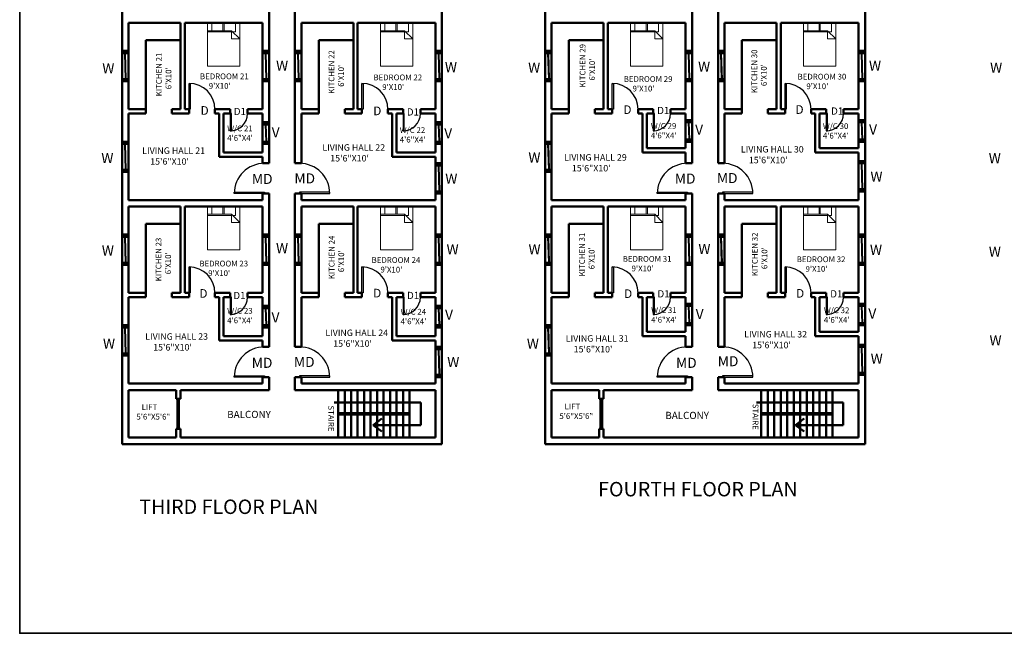
# Model space of a CAD drawing. Units: inches. Extents: x 9239 to 26065, y 6728 to 14611.
# Tile 7 of 12: x 23324 to 24691, y 11592 to 12444. Entities that reach past the tile are written whole.
import ezdxf

# ---------------------------------------------------------------- set-up
doc = ezdxf.new("R2010")
doc.units = ezdxf.units.IN
doc.header["$MEASUREMENT"] = 0
for name, color, linetype, lineweight in [('A-ANNO-TEXT', 7, 'Continuous', 18), ('A-ANNO-TTLB', 7, 'Continuous', 35), ('A-AREA-IDEN', 7, 'Continuous', 18), ('A-DOOR', 4, 'Continuous', 25), ('A-FURN', 8, 'Continuous', 18), ('A-GLAZ', 4, 'Continuous', 25), ('A-WALL', 7, 'Continuous', 50)]:
    doc.layers.add(name, color=color, linetype=linetype, lineweight=lineweight)
doc.styles.get("Standard").update_dxf_attribs({"font": 'arial.ttf'})

# ---------------------------------------------------------------- blocks, each defined once
blk = doc.blocks.new('*U10')
for p, q in [((0, 0), (0, -6)), ((36, 0), (36, -6))]:
    blk.add_line(p, q)
blk.add_lwpolyline([(0, 0), (0, 36), (1.75, 36), (1.75, 0)], close=True)
blk.add_arc((0, 0), 36, 0, 90)
blk = doc.blocks.new('*U34')
for p, q in [((0, 0), (0, 6)), ((24, 0), (24, 6))]:
    blk.add_line(p, q)
blk.add_lwpolyline([(0, 0), (0, -24), (1.75, -24), (1.75, 0)], close=True)
blk.add_arc((0, 0), 24, 270, 0)
blk = doc.blocks.new('*U33')
for p, q in [((-40, 0), (-40, 6)), ((0, 0), (0, 6))]:
    blk.add_line(p, q)
blk.add_lwpolyline([(0, 0), (0, -40), (-1.75, -40), (-1.75, 0)], close=True)
blk.add_arc((0, 0), 40, 180, 270)
blk = doc.blocks.new('*U35')
for p, q in [((0, 0), (0, -6)), ((-40, 0), (-40, -6))]:
    blk.add_line(p, q)
blk.add_lwpolyline([(0, 0), (0, 40), (-1.75, 40), (-1.75, 0)], close=True)
blk.add_arc((0, 0), 40, 90, 180)
blk = doc.blocks.new('Bed - Queen')
for p, q in [((0, -80.00003), (0, 0)), ((0, 0), (59.99999, 0)), ((59.99999, 0), (59.99999, -80.00003)), ((0, -14.4), (44.8, -14.4)), ((44.8, -16.8), (0, -16.8)), ((7.99999, -1.2), (28.79998, -1.2)), ((7.99999, -14.4), (7.99999, -1.2)), ((28.79998, -1.2), (28.79998, -14.4)), ((31.19999, -1.2), (51.99999, -1.2)), ((31.19999, -14.4), (31.19999, -1.2)), ((59.99999, -29.6), (44.8, -14.4)), ((44.8, -14.4), (44.8, -29.6)), ((51.99999, -16.4), (46.79936, -16.4)), ((51.99999, -1.2), (51.99999, -16.4)), ((44.8, -29.6), (59.99999, -29.6)), ((59.99999, -80.00003), (0, -80.00003))]:
    blk.add_line(p, q)
blk = doc.blocks.new('WIN-36')
for p, q in [((0, 1), (36, 1)), ((0, 0.5), (36, 0.5)), ((0, 0), (36, 0))]:
    blk.add_line(p, q)
blk = doc.blocks.new('WIN-24')
for p, q in [((0, 1), (24, 1)), ((0, 0.5), (24, 0.5)), ((0, 0), (24, 0))]:
    blk.add_line(p, q)

msp = doc.modelspace()

# ---------------------------------------------------------------- linework, layer by layer
at = {"layer": 'A-ANNO-TTLB'}
msp.add_lwpolyline([(23324.14, 14611.25), (26064.6, 14611.25), (26064.6, 11591.84), (23324.14, 11591.84)], close=True, dxfattribs=at)
at = {"layer": 'A-WALL'}
for p, q in [((23466.16, 11854.64), (23466.16, 12958.64)), ((23910.16, 12958.64), (23910.16, 11854.64)), ((24053.28, 11854.64), (24053.28, 12958.64)), ((24497.28, 12958.64), (24497.28, 11854.64)), ((23670.16, 12244.64), (23670.16, 12457.64)), ((23706.16, 12457.64), (23706.16, 12244.64)), ((24257.28, 12244.64), (24257.28, 12457.64)), ((24293.28, 12457.64), (24293.28, 12244.64)), ((23475.16, 12439.64), (23547.16, 12439.64)), ((23475.16, 12319.64), (23475.16, 12439.64)), ((23547.16, 12319.64), (23547.16, 12439.64)), ((23553.16, 12319.64), (23553.16, 12439.64)), ((23553.16, 12439.64), (23661.16, 12439.64)), ((23661.16, 12319.64), (23661.16, 12439.64)), ((23715.16, 12439.64), (23787.16, 12439.64)), ((23715.16, 12439.64), (23715.16, 12319.64)), ((23787.16, 12439.64), (23787.16, 12319.64)), ((23793.16, 12439.64), (23793.16, 12319.64)), ((23793.16, 12439.64), (23901.16, 12439.64)), ((23901.16, 12439.64), (23901.16, 12319.64)), ((24062.28, 12439.64), (24134.28, 12439.64)), ((24062.28, 12319.64), (24062.28, 12439.64)), ((24134.28, 12319.64), (24134.28, 12439.64)), ((24140.28, 12319.64), (24140.28, 12439.64)), ((24140.28, 12439.64), (24248.28, 12439.64)), ((24248.28, 12319.64), (24248.28, 12439.64)), ((24302.28, 12439.64), (24374.28, 12439.64)), ((24302.28, 12439.64), (24302.28, 12319.64)), ((24374.28, 12439.64), (24374.28, 12319.64)), ((24380.28, 12439.64), (24380.28, 12319.64)), ((24380.28, 12439.64), (24488.28, 12439.64)), ((24488.28, 12439.64), (24488.28, 12319.64)), ((23499.16, 12319.64), (23499.16, 12415.64)), ((23499.16, 12415.64), (23547.16, 12415.64)), ((23739.16, 12415.64), (23739.16, 12319.64)), ((23739.16, 12415.64), (23787.16, 12415.64)), ((24086.28, 12319.64), (24086.28, 12415.64)), ((24086.28, 12415.64), (24134.28, 12415.64)), ((24326.28, 12415.64), (24326.28, 12319.64)), ((24326.28, 12415.64), (24374.28, 12415.64)), ((23475.16, 12400.64), (23466.16, 12400.64)), ((23475.16, 12397.64), (23466.16, 12397.64)), ((23661.16, 12400.64), (23670.16, 12400.64)), ((23661.16, 12397.64), (23670.16, 12397.64)), ((23715.16, 12400.64), (23706.16, 12400.64)), ((23715.16, 12397.64), (23706.16, 12397.64)), ((23901.16, 12400.64), (23910.16, 12400.64)), ((23901.16, 12397.64), (23910.16, 12397.64)), ((24062.28, 12400.64), (24053.28, 12400.64)), ((24062.28, 12397.64), (24053.28, 12397.64)), ((24248.28, 12400.64), (24257.28, 12400.64)), ((24248.28, 12397.64), (24257.28, 12397.64)), ((24302.28, 12400.64), (24293.28, 12400.64)), ((24302.28, 12397.64), (24293.28, 12397.64)), ((24488.28, 12400.64), (24497.28, 12400.64)), ((24488.28, 12397.64), (24497.28, 12397.64)), ((23475.16, 12361.64), (23466.16, 12361.64)), ((23475.16, 12358.64), (23466.16, 12358.64)), ((23661.16, 12361.64), (23670.16, 12361.64)), ((23661.16, 12358.64), (23670.16, 12358.64)), ((23715.16, 12361.64), (23706.16, 12361.64)), ((23715.16, 12358.64), (23706.16, 12358.64)), ((23901.16, 12361.64), (23910.16, 12361.64)), ((23901.16, 12358.64), (23910.16, 12358.64)), ((24062.28, 12361.64), (24053.28, 12361.64)), ((24062.28, 12358.64), (24053.28, 12358.64)), ((24248.28, 12361.64), (24257.28, 12361.64)), ((24248.28, 12358.64), (24257.28, 12358.64)), ((24302.28, 12361.64), (24293.28, 12361.64)), ((24302.28, 12358.64), (24293.28, 12358.64)), ((24488.28, 12361.64), (24497.28, 12361.64)), ((24488.28, 12358.64), (24497.28, 12358.64)), ((23475.16, 12319.64), (23499.16, 12319.64)), ((23475.16, 12313.64), (23499.16, 12313.64)), ((23475.16, 12193.64), (23475.16, 12313.64)), ((23499.16, 12313.64), (23499.16, 12319.64)), ((23535.16, 12313.64), (23535.16, 12319.64)), ((23535.16, 12319.64), (23547.16, 12319.64)), ((23535.16, 12313.64), (23559.16, 12313.64)), ((23553.16, 12319.64), (23559.16, 12319.64)), ((23559.16, 12313.64), (23559.16, 12319.64)), ((23595.16, 12313.64), (23595.16, 12319.64)), ((23595.16, 12319.64), (23616.16, 12319.64)), ((23595.16, 12313.64), (23601.16, 12313.64)), ((23601.16, 12253.64), (23601.16, 12313.64)), ((23607.16, 12259.64), (23607.16, 12313.64)), ((23607.16, 12313.64), (23616.16, 12313.64)), ((23616.16, 12313.64), (23616.16, 12319.64)), ((23640.16, 12313.64), (23640.16, 12319.64)), ((23640.16, 12319.64), (23661.16, 12319.64)), ((23640.16, 12313.64), (23661.16, 12313.64)), ((23661.16, 12259.64), (23661.16, 12313.64)), ((23715.16, 12319.64), (23739.16, 12319.64)), ((23715.16, 12313.64), (23739.16, 12313.64)), ((23715.16, 12313.64), (23715.16, 12244.64)), ((23739.16, 12319.64), (23739.16, 12313.64)), ((23775.16, 12319.64), (23775.16, 12313.64)), ((23775.16, 12319.64), (23787.16, 12319.64)), ((23775.16, 12313.64), (23799.16, 12313.64)), ((23793.16, 12319.64), (23799.16, 12319.64)), ((23799.16, 12319.64), (23799.16, 12313.64)), ((23835.16, 12319.64), (23835.16, 12313.64)), ((23835.16, 12319.64), (23856.16, 12319.64)), ((23835.16, 12313.64), (23841.16, 12313.64)), ((23841.16, 12313.64), (23841.16, 12253.64)), ((23847.16, 12313.64), (23847.16, 12259.64)), ((23847.16, 12313.64), (23856.16, 12313.64)), ((23856.16, 12319.64), (23856.16, 12313.64)), ((23880.16, 12319.64), (23880.16, 12313.64)), ((23880.16, 12319.64), (23901.16, 12319.64)), ((23880.16, 12313.64), (23901.16, 12313.64)), ((23901.16, 12313.64), (23901.16, 12259.64)), ((24062.28, 12319.64), (24086.28, 12319.64)), ((24062.28, 12313.64), (24086.28, 12313.64)), ((24062.28, 12193.64), (24062.28, 12313.64)), ((24086.28, 12313.64), (24086.28, 12319.64)), ((24122.28, 12313.64), (24122.28, 12319.64)), ((24122.28, 12319.64), (24134.28, 12319.64)), ((24122.28, 12313.64), (24146.28, 12313.64)), ((24140.28, 12319.64), (24146.28, 12319.64)), ((24146.28, 12313.64), (24146.28, 12319.64)), ((24182.28, 12313.64), (24182.28, 12319.64)), ((24182.28, 12319.64), (24203.28, 12319.64)), ((24182.28, 12313.64), (24188.28, 12313.64)), ((24188.28, 12259.64), (24188.28, 12313.64)), ((24194.28, 12265.64), (24194.28, 12313.64)), ((24194.28, 12313.64), (24203.28, 12313.64)), ((24203.28, 12313.64), (24203.28, 12319.64)), ((24227.28, 12313.64), (24227.28, 12319.64)), ((24227.28, 12319.64), (24248.28, 12319.64)), ((24227.28, 12313.64), (24248.28, 12313.64)), ((24248.28, 12265.64), (24248.28, 12313.64)), ((24302.28, 12319.64), (24326.28, 12319.64)), ((24302.28, 12313.64), (24326.28, 12313.64)), ((24302.28, 12313.64), (24302.28, 12244.64)), ((24326.28, 12319.64), (24326.28, 12313.64)), ((24362.28, 12319.64), (24362.28, 12313.64)), ((24362.28, 12319.64), (24374.28, 12319.64)), ((24362.28, 12313.64), (24386.28, 12313.64)), ((24380.28, 12319.64), (24386.28, 12319.64)), ((24386.28, 12319.64), (24386.28, 12313.64)), ((24422.28, 12319.64), (24422.28, 12313.64)), ((24422.28, 12319.64), (24443.28, 12319.64)), ((24422.28, 12313.64), (24428.28, 12313.64)), ((24428.28, 12313.64), (24428.28, 12259.64)), ((24434.28, 12313.64), (24434.28, 12265.64)), ((24434.28, 12313.64), (24443.28, 12313.64)), ((24443.28, 12319.64), (24443.28, 12313.64)), ((24467.28, 12319.64), (24467.28, 12313.64)), ((24467.28, 12319.64), (24488.28, 12319.64)), ((24467.28, 12313.64), (24488.28, 12313.64)), ((24488.28, 12313.64), (24488.28, 12265.64)), ((23661.16, 12301.64), (23670.16, 12301.64)), ((23661.16, 12298.64), (23670.16, 12298.64)), ((23901.16, 12301.64), (23910.16, 12301.64)), ((23901.16, 12298.64), (23910.16, 12298.64)), ((24248.28, 12304.64), (24257.28, 12304.64)), ((24248.28, 12301.64), (24257.28, 12301.64)), ((24488.28, 12304.64), (24497.28, 12304.64)), ((24488.28, 12301.64), (24497.28, 12301.64)), ((23475.16, 12274.64), (23466.16, 12274.64)), ((23475.16, 12271.64), (23466.16, 12271.64)), ((23661.16, 12274.64), (23670.16, 12274.64)), ((23661.16, 12271.64), (23670.16, 12271.64)), ((23901.16, 12274.64), (23910.16, 12274.64)), ((23901.16, 12271.64), (23910.16, 12271.64)), ((24062.28, 12274.64), (24053.28, 12274.64)), ((24062.28, 12271.64), (24053.28, 12271.64)), ((24248.28, 12277.64), (24257.28, 12277.64)), ((24248.28, 12274.64), (24257.28, 12274.64)), ((24488.28, 12277.64), (24497.28, 12277.64)), ((24488.28, 12274.64), (24497.28, 12274.64)), ((23607.16, 12259.64), (23661.16, 12259.64)), ((23847.16, 12259.64), (23901.16, 12259.64)), ((24188.28, 12259.64), (24248.28, 12259.64)), ((24194.28, 12265.64), (24248.28, 12265.64)), ((24248.28, 12244.64), (24248.28, 12259.64)), ((24428.28, 12259.64), (24488.28, 12259.64)), ((24434.28, 12265.64), (24488.28, 12265.64)), ((24488.28, 12259.64), (24488.28, 12193.64)), ((23601.16, 12253.64), (23661.16, 12253.64)), ((23661.16, 12244.64), (23661.16, 12253.64)), ((23661.16, 12244.64), (23670.16, 12244.64)), ((23706.16, 12244.64), (23715.16, 12244.64)), ((23841.16, 12253.64), (23901.16, 12253.64)), ((23901.16, 12253.64), (23901.16, 12193.64)), ((23901.16, 12244.64), (23910.16, 12244.64)), ((24248.28, 12244.64), (24257.28, 12244.64)), ((24293.28, 12244.64), (24302.28, 12244.64)), ((24488.28, 12247.64), (24497.28, 12247.64)), ((24488.28, 12244.64), (24497.28, 12244.64)), ((23475.16, 12235.64), (23466.16, 12235.64)), ((23475.16, 12232.64), (23466.16, 12232.64)), ((23901.16, 12241.64), (23910.16, 12241.64)), ((24062.28, 12235.64), (24053.28, 12235.64)), ((24062.28, 12232.64), (24053.28, 12232.64)), ((23661.16, 12202.64), (23670.16, 12202.64)), ((23661.16, 12193.64), (23661.16, 12202.64)), ((23670.16, 11989.64), (23670.16, 12202.64)), ((23706.16, 12202.64), (23715.16, 12202.64)), ((23706.16, 12202.64), (23706.16, 11989.64)), ((23715.16, 12202.64), (23715.16, 12193.64)), ((23901.16, 12205.64), (23910.16, 12205.64)), ((23901.16, 12202.64), (23910.16, 12202.64)), ((24248.28, 12202.64), (24257.28, 12202.64)), ((24248.28, 12193.64), (24248.28, 12202.64)), ((24257.28, 11989.64), (24257.28, 12202.64)), ((24293.28, 12202.64), (24302.28, 12202.64)), ((24293.28, 12202.64), (24293.28, 11989.64)), ((24302.28, 12202.64), (24302.28, 12193.64)), ((24488.28, 12208.64), (24497.28, 12208.64)), ((24488.28, 12205.64), (24497.28, 12205.64)), ((23475.16, 12193.64), (23661.16, 12193.64)), ((23715.16, 12193.64), (23901.16, 12193.64)), ((24062.28, 12193.64), (24248.28, 12193.64)), ((24302.28, 12193.64), (24488.28, 12193.64)), ((23475.16, 12184.64), (23547.16, 12184.64)), ((23475.16, 12064.64), (23475.16, 12184.64)), ((23547.16, 12064.64), (23547.16, 12184.64)), ((23553.16, 12064.64), (23553.16, 12184.64)), ((23553.16, 12184.64), (23661.16, 12184.64)), ((23661.16, 12064.64), (23661.16, 12184.64)), ((23715.16, 12184.64), (23787.16, 12184.64)), ((23715.16, 12184.64), (23715.16, 12064.64)), ((23787.16, 12184.64), (23787.16, 12064.64)), ((23793.16, 12184.64), (23793.16, 12064.64)), ((23793.16, 12184.64), (23901.16, 12184.64)), ((23901.16, 12184.64), (23901.16, 12064.64)), ((24062.28, 12184.64), (24134.28, 12184.64)), ((24062.28, 12064.64), (24062.28, 12184.64)), ((24134.28, 12064.64), (24134.28, 12184.64)), ((24140.28, 12064.64), (24140.28, 12184.64)), ((24140.28, 12184.64), (24248.28, 12184.64)), ((24248.28, 12064.64), (24248.28, 12184.64)), ((24302.28, 12184.64), (24374.28, 12184.64)), ((24302.28, 12184.64), (24302.28, 12064.64)), ((24374.28, 12184.64), (24374.28, 12064.64)), ((24380.28, 12184.64), (24380.28, 12064.64)), ((24380.28, 12184.64), (24488.28, 12184.64)), ((24488.28, 12184.64), (24488.28, 12064.64)), ((23499.16, 12064.64), (23499.16, 12160.64)), ((23499.16, 12160.64), (23547.16, 12160.64)), ((23739.16, 12160.64), (23739.16, 12064.64)), ((23739.16, 12160.64), (23787.16, 12160.64)), ((24086.28, 12064.64), (24086.28, 12160.64)), ((24086.28, 12160.64), (24134.28, 12160.64)), ((24326.28, 12160.64), (24326.28, 12064.64)), ((24326.28, 12160.64), (24374.28, 12160.64)), ((23475.16, 12145.64), (23466.16, 12145.64)), ((23475.16, 12142.64), (23466.16, 12142.64)), ((23661.16, 12145.64), (23670.16, 12145.64)), ((23661.16, 12142.64), (23670.16, 12142.64)), ((23715.16, 12145.64), (23706.16, 12145.64)), ((23715.16, 12142.64), (23706.16, 12142.64)), ((23901.16, 12145.64), (23910.16, 12145.64)), ((23901.16, 12142.64), (23910.16, 12142.64)), ((24062.28, 12145.64), (24053.28, 12145.64)), ((24062.28, 12142.64), (24053.28, 12142.64)), ((24248.28, 12145.64), (24257.28, 12145.64)), ((24248.28, 12142.64), (24257.28, 12142.64)), ((24302.28, 12145.64), (24293.28, 12145.64)), ((24302.28, 12142.64), (24293.28, 12142.64)), ((24488.28, 12145.64), (24497.28, 12145.64)), ((24488.28, 12142.64), (24497.28, 12142.64)), ((23475.16, 12106.64), (23466.16, 12106.64)), ((23661.16, 12106.64), (23670.16, 12106.64)), ((23715.16, 12106.64), (23706.16, 12106.64)), ((23901.16, 12106.64), (23910.16, 12106.64)), ((24062.28, 12106.64), (24053.28, 12106.64)), ((24248.28, 12106.64), (24257.28, 12106.64)), ((24302.28, 12106.64), (24293.28, 12106.64)), ((24488.28, 12106.64), (24497.28, 12106.64)), ((23475.16, 12103.64), (23466.16, 12103.64)), ((23661.16, 12103.64), (23670.16, 12103.64)), ((23715.16, 12103.64), (23706.16, 12103.64)), ((23901.16, 12103.64), (23910.16, 12103.64)), ((24062.28, 12103.64), (24053.28, 12103.64)), ((24248.28, 12103.64), (24257.28, 12103.64)), ((24302.28, 12103.64), (24293.28, 12103.64)), ((24488.28, 12103.64), (24497.28, 12103.64)), ((23475.16, 12064.64), (23499.16, 12064.64)), ((23475.16, 12058.64), (23499.16, 12058.64)), ((23475.16, 11938.64), (23475.16, 12058.64)), ((23499.16, 12058.64), (23499.16, 12064.64)), ((23535.16, 12058.64), (23535.16, 12064.64)), ((23535.16, 12064.64), (23547.16, 12064.64)), ((23535.16, 12058.64), (23559.16, 12058.64)), ((23553.16, 12064.64), (23559.16, 12064.64)), ((23559.16, 12058.64), (23559.16, 12064.64)), ((23595.16, 12058.64), (23595.16, 12064.64)), ((23595.16, 12064.64), (23616.16, 12064.64)), ((23595.16, 12058.64), (23601.16, 12058.64)), ((23601.16, 11998.64), (23601.16, 12058.64)), ((23607.16, 12004.64), (23607.16, 12058.64)), ((23607.16, 12058.64), (23616.16, 12058.64)), ((23616.16, 12058.64), (23616.16, 12064.64)), ((23640.16, 12058.64), (23640.16, 12064.64)), ((23640.16, 12064.64), (23661.16, 12064.64)), ((23640.16, 12058.64), (23661.16, 12058.64)), ((23661.16, 12004.64), (23661.16, 12058.64)), ((23715.16, 12064.64), (23739.16, 12064.64)), ((23715.16, 12058.64), (23739.16, 12058.64)), ((23715.16, 12058.64), (23715.16, 11989.64)), ((23739.16, 12064.64), (23739.16, 12058.64)), ((23775.16, 12064.64), (23775.16, 12058.64)), ((23775.16, 12064.64), (23787.16, 12064.64)), ((23775.16, 12058.64), (23799.16, 12058.64)), ((23793.16, 12064.64), (23799.16, 12064.64)), ((23799.16, 12064.64), (23799.16, 12058.64)), ((23835.16, 12064.64), (23835.16, 12058.64)), ((23835.16, 12064.64), (23856.16, 12064.64)), ((23835.16, 12058.64), (23841.16, 12058.64)), ((23841.16, 12058.64), (23841.16, 11998.64)), ((23847.16, 12058.64), (23847.16, 12004.64)), ((23847.16, 12058.64), (23856.16, 12058.64)), ((23856.16, 12064.64), (23856.16, 12058.64)), ((23880.16, 12064.64), (23880.16, 12058.64)), ((23880.16, 12064.64), (23901.16, 12064.64)), ((23880.16, 12058.64), (23901.16, 12058.64)), ((23901.16, 12058.64), (23901.16, 12004.64)), ((24062.28, 12064.64), (24086.28, 12064.64)), ((24062.28, 12058.64), (24086.28, 12058.64)), ((24062.28, 11938.64), (24062.28, 12058.64)), ((24086.28, 12058.64), (24086.28, 12064.64)), ((24122.28, 12058.64), (24122.28, 12064.64)), ((24122.28, 12064.64), (24134.28, 12064.64)), ((24122.28, 12058.64), (24146.28, 12058.64)), ((24140.28, 12064.64), (24146.28, 12064.64)), ((24146.28, 12058.64), (24146.28, 12064.64)), ((24182.28, 12058.64), (24182.28, 12064.64)), ((24182.28, 12064.64), (24203.28, 12064.64)), ((24182.28, 12058.64), (24188.28, 12058.64)), ((24188.28, 12004.64), (24188.28, 12058.64)), ((24194.28, 12010.64), (24194.28, 12058.64)), ((24194.28, 12058.64), (24203.28, 12058.64)), ((24203.28, 12058.64), (24203.28, 12064.64)), ((24227.28, 12058.64), (24227.28, 12064.64)), ((24227.28, 12064.64), (24248.28, 12064.64)), ((24227.28, 12058.64), (24248.28, 12058.64)), ((24248.28, 12010.64), (24248.28, 12058.64)), ((24302.28, 12064.64), (24326.28, 12064.64)), ((24302.28, 12058.64), (24326.28, 12058.64)), ((24302.28, 12058.64), (24302.28, 11989.64)), ((24326.28, 12064.64), (24326.28, 12058.64)), ((24362.28, 12064.64), (24362.28, 12058.64)), ((24362.28, 12064.64), (24374.28, 12064.64)), ((24362.28, 12058.64), (24386.28, 12058.64)), ((24380.28, 12064.64), (24386.28, 12064.64)), ((24386.28, 12064.64), (24386.28, 12058.64)), ((24422.28, 12064.64), (24422.28, 12058.64)), ((24422.28, 12064.64), (24443.28, 12064.64)), ((24422.28, 12058.64), (24428.28, 12058.64)), ((24428.28, 12058.64), (24428.28, 12004.64)), ((24434.28, 12058.64), (24434.28, 12010.64)), ((24434.28, 12058.64), (24443.28, 12058.64)), ((24443.28, 12064.64), (24443.28, 12058.64)), ((24467.28, 12064.64), (24467.28, 12058.64)), ((24467.28, 12064.64), (24488.28, 12064.64)), ((24467.28, 12058.64), (24488.28, 12058.64)), ((24488.28, 12058.64), (24488.28, 12010.64)), ((23661.16, 12046.64), (23670.16, 12046.64)), ((23661.16, 12043.64), (23670.16, 12043.64)), ((23901.16, 12046.64), (23910.16, 12046.64)), ((23901.16, 12043.64), (23910.16, 12043.64)), ((24248.28, 12049.64), (24257.28, 12049.64)), ((24248.28, 12046.64), (24257.28, 12046.64)), ((24488.28, 12049.64), (24497.28, 12049.64)), ((24488.28, 12046.64), (24497.28, 12046.64)), ((23475.16, 12019.64), (23466.16, 12019.64)), ((23475.16, 12016.64), (23466.16, 12016.64)), ((23661.16, 12019.64), (23670.16, 12019.64)), ((23661.16, 12016.64), (23670.16, 12016.64)), ((23901.16, 12019.64), (23910.16, 12019.64)), ((23901.16, 12016.64), (23910.16, 12016.64)), ((24062.28, 12019.64), (24053.28, 12019.64)), ((24062.28, 12016.64), (24053.28, 12016.64)), ((24194.28, 12010.64), (24248.28, 12010.64)), ((24248.28, 12022.64), (24257.28, 12022.64)), ((24248.28, 12019.64), (24257.28, 12019.64)), ((24434.28, 12010.64), (24488.28, 12010.64)), ((24488.28, 12022.64), (24497.28, 12022.64)), ((24488.28, 12019.64), (24497.28, 12019.64)), ((23601.16, 11998.64), (23661.16, 11998.64)), ((23607.16, 12004.64), (23661.16, 12004.64)), ((23661.16, 11989.64), (23661.16, 11998.64)), ((23841.16, 11998.64), (23901.16, 11998.64)), ((23847.16, 12004.64), (23901.16, 12004.64)), ((23901.16, 11998.64), (23901.16, 11938.64)), ((24188.28, 12004.64), (24248.28, 12004.64)), ((24248.28, 11989.64), (24248.28, 12004.64)), ((24428.28, 12004.64), (24488.28, 12004.64)), ((24488.28, 12004.64), (24488.28, 11938.64)), ((23661.16, 11989.64), (23670.16, 11989.64)), ((23706.16, 11989.64), (23715.16, 11989.64)), ((23901.16, 11989.64), (23910.16, 11989.64)), ((23901.16, 11986.64), (23910.16, 11986.64)), ((24248.28, 11989.64), (24257.28, 11989.64)), ((24293.28, 11989.64), (24302.28, 11989.64)), ((24488.28, 11992.64), (24497.28, 11992.64)), ((24488.28, 11989.64), (24497.28, 11989.64)), ((23475.16, 11980.64), (23466.16, 11980.64)), ((23475.16, 11977.64), (23466.16, 11977.64)), ((24062.28, 11980.64), (24053.28, 11980.64)), ((24062.28, 11977.64), (24053.28, 11977.64)), ((23661.16, 11938.64), (23661.16, 11947.64)), ((23661.16, 11947.64), (23670.16, 11947.64)), ((23670.16, 11929.64), (23670.16, 11947.64)), ((23706.16, 11947.64), (23715.16, 11947.64)), ((23706.16, 11947.64), (23706.16, 11929.64)), ((23715.16, 11947.64), (23715.16, 11938.64)), ((23901.16, 11950.64), (23910.16, 11950.64)), ((23901.16, 11947.64), (23910.16, 11947.64)), ((24248.28, 11938.64), (24248.28, 11947.64)), ((24248.28, 11947.64), (24257.28, 11947.64)), ((24257.28, 11929.64), (24257.28, 11947.64)), ((24293.28, 11947.64), (24302.28, 11947.64)), ((24293.28, 11947.64), (24293.28, 11929.64)), ((24302.28, 11947.64), (24302.28, 11938.64)), ((24488.28, 11953.64), (24497.28, 11953.64)), ((24488.28, 11950.64), (24497.28, 11950.64)), ((23475.16, 11938.64), (23661.16, 11938.64)), ((23475.16, 11863.64), (23475.16, 11929.64)), ((23475.16, 11929.64), (23541.16, 11929.64)), ((23541.16, 11917.64), (23541.16, 11929.64)), ((23547.16, 11929.64), (23670.16, 11929.64)), ((23547.16, 11917.64), (23547.16, 11929.64)), ((23706.16, 11929.64), (23901.16, 11929.64)), ((23715.16, 11938.64), (23901.16, 11938.64)), ((23766.16, 11929.64), (23766.16, 11863.64)), ((23775.16, 11929.64), (23775.16, 11897.64)), ((23784.16, 11929.64), (23784.16, 11897.64)), ((23793.16, 11929.64), (23793.16, 11897.64)), ((23802.16, 11929.64), (23802.16, 11897.64)), ((23811.16, 11929.64), (23811.16, 11897.64)), ((23820.16, 11929.64), (23820.16, 11897.64)), ((23829.16, 11929.64), (23829.16, 11897.64)), ((23838.16, 11929.64), (23838.16, 11897.64)), ((23847.16, 11929.64), (23847.16, 11897.64)), ((23856.16, 11929.64), (23856.16, 11897.64)), ((23865.16, 11929.64), (23865.16, 11863.64)), ((23901.16, 11929.64), (23901.16, 11863.64)), ((24062.28, 11938.64), (24248.28, 11938.64)), ((24062.28, 11863.64), (24062.28, 11929.64)), ((24062.28, 11929.64), (24128.28, 11929.64)), ((24128.28, 11917.64), (24128.28, 11929.64)), ((24134.28, 11929.64), (24257.28, 11929.64)), ((24134.28, 11917.64), (24134.28, 11929.64)), ((24293.28, 11929.64), (24488.28, 11929.64)), ((24302.28, 11938.64), (24488.28, 11938.64)), ((24353.28, 11929.64), (24353.28, 11863.64)), ((24362.28, 11929.64), (24362.28, 11897.64)), ((24371.28, 11929.64), (24371.28, 11897.64)), ((24380.28, 11929.64), (24380.28, 11897.64)), ((24389.28, 11929.64), (24389.28, 11897.64)), ((24398.28, 11929.64), (24398.28, 11897.64)), ((24407.28, 11929.64), (24407.28, 11897.64)), ((24416.28, 11929.64), (24416.28, 11897.64)), ((24425.28, 11929.64), (24425.28, 11897.64)), ((24434.28, 11929.64), (24434.28, 11897.64)), ((24443.28, 11929.64), (24443.28, 11897.64)), ((24452.28, 11929.64), (24452.28, 11863.64)), ((24488.28, 11929.64), (24488.28, 11863.64)), ((23541.16, 11917.64), (23547.16, 11917.64)), ((23543.16, 11917.64), (23543.16, 11875.64)), ((23545.16, 11917.64), (23545.16, 11875.64)), ((24128.28, 11917.64), (24134.28, 11917.64)), ((24130.28, 11917.64), (24130.28, 11875.64)), ((24132.28, 11917.64), (24132.28, 11875.64)), ((23760.52, 11912.46), (23880.96, 11912.46)), ((23880.96, 11912.46), (23880.96, 11880.96)), ((24346.71, 11912.46), (24467.14, 11912.46)), ((24467.14, 11912.46), (24467.14, 11880.96)), ((23766.16, 11897.64), (23865.16, 11897.64)), ((23766.16, 11895.64), (23865.16, 11895.64)), ((23775.16, 11895.64), (23775.16, 11863.64)), ((23784.16, 11895.64), (23784.16, 11863.64)), ((23793.16, 11895.64), (23793.16, 11863.64)), ((23802.16, 11895.64), (23802.16, 11863.64)), ((23811.16, 11895.64), (23811.16, 11863.64)), ((23814.75, 11880.96), (23826.81, 11890.22)), ((23820.16, 11895.64), (23820.16, 11863.64)), ((23829.16, 11895.64), (23829.16, 11863.64)), ((23838.16, 11895.64), (23838.16, 11863.64)), ((23847.16, 11895.64), (23847.16, 11863.64)), ((23856.16, 11895.64), (23856.16, 11863.64)), ((24353.28, 11897.64), (24452.28, 11897.64)), ((24353.28, 11895.64), (24452.28, 11895.64)), ((24362.28, 11895.64), (24362.28, 11863.64)), ((24371.28, 11895.64), (24371.28, 11863.64)), ((24380.28, 11895.64), (24380.28, 11863.64)), ((24389.28, 11895.64), (24389.28, 11863.64)), ((24398.28, 11895.64), (24398.28, 11863.64)), ((24400.93, 11880.96), (24413, 11890.22)), ((24407.28, 11895.64), (24407.28, 11863.64)), ((24416.28, 11895.64), (24416.28, 11863.64)), ((24425.28, 11895.64), (24425.28, 11863.64)), ((24434.28, 11895.64), (24434.28, 11863.64)), ((24443.28, 11895.64), (24443.28, 11863.64)), ((23541.16, 11863.64), (23541.16, 11875.64)), ((23547.16, 11875.64), (23541.16, 11875.64)), ((23547.16, 11863.64), (23547.16, 11875.64)), ((23880.96, 11880.96), (23814.75, 11880.96)), ((23814.75, 11880.96), (23826.52, 11872.2)), ((24128.28, 11863.64), (24128.28, 11875.64)), ((24134.28, 11875.64), (24128.28, 11875.64)), ((24134.28, 11863.64), (24134.28, 11875.64)), ((24467.14, 11880.96), (24400.93, 11880.96)), ((24400.93, 11880.96), (24412.71, 11872.2)), ((23541.16, 11863.64), (23475.16, 11863.64)), ((23901.16, 11863.64), (23547.16, 11863.64)), ((24128.28, 11863.64), (24062.28, 11863.64)), ((24488.28, 11863.64), (24134.28, 11863.64)), ((23910.16, 11854.64), (23466.16, 11854.64)), ((24497.28, 11854.64), (24053.28, 11854.64))]:
    msp.add_line(p, q, dxfattribs=at)

# ---------------------------------------------------------------- block references
at = {"layer": 'A-DOOR'}
for name, p in [('*U10', (23559.16, 12319.64)), ('*U10', (23799.16, 12319.64)), ('*U10', (24146.28, 12319.64)), ('*U10', (24386.28, 12319.64)), ('*U34', (23616.16, 12313.64)), ('*U34', (23856.16, 12313.64)), ('*U34', (24203.28, 12313.64)), ('*U34', (24443.28, 12313.64)), ('*U10', (23559.16, 12064.64)), ('*U10', (23799.16, 12064.64)), ('*U10', (24146.28, 12064.64)), ('*U10', (24386.28, 12064.64)), ('*U34', (23616.16, 12058.64)), ('*U34', (23856.16, 12058.64)), ('*U34', (24203.28, 12058.64)), ('*U34', (24443.28, 12058.64))]:
    msp.add_blockref(name, p, dxfattribs=at)
at = {"layer": 'A-DOOR', "xscale": 1.05, "yscale": 1.05, "zscale": 1.05, "rotation": 270}
for name, p in [('*U33', (23663.86, 12202.64)), ('*U35', (23712.46, 12202.64)), ('*U33', (24250.98, 12202.64)), ('*U35', (24299.58, 12202.64)), ('*U33', (23663.86, 11947.64)), ('*U35', (23712.46, 11947.64)), ('*U33', (24250.98, 11947.64)), ('*U35', (24299.58, 11947.64))]:
    msp.add_blockref(name, p, dxfattribs=at)
at = {"layer": 'A-FURN', "xscale": 0.75, "yscale": 0.75, "zscale": 0.75}
for p in [(23584.66, 12439.64), (23824.66, 12439.64), (24171.78, 12439.64), (24411.78, 12439.64), (23584.66, 12184.64), (23824.66, 12184.64), (24171.78, 12184.64), (24411.78, 12184.64)]:
    msp.add_blockref('Bed - Queen', p, dxfattribs=at)
at = {"layer": 'A-GLAZ'}
for name, p, rotation in [('WIN-36', (23469.66, 12397.62), 271.5911402712003), ('WIN-36', (23664.66, 12397.62), 271.5911402711888), ('WIN-36', (23709.66, 12397.62), 271.5911402711888), ('WIN-36', (23904.66, 12397.62), 271.5911402711888), ('WIN-36', (24056.78, 12397.62), 271.5911402712003), ('WIN-36', (24251.78, 12397.62), 271.5911402712235), ('WIN-36', (24296.78, 12397.62), 271.5911402712003), ('WIN-36', (24491.78, 12397.62), 271.5911402712003), ('WIN-24', (23664.66, 12298.61), 272.3859440303801), ('WIN-24', (23904.66, 12298.61), 272.3859440303801), ('WIN-24', (24251.78, 12301.61), 272.3859440303975), ('WIN-24', (24491.78, 12301.61), 272.3859440303975), ('WIN-36', (23469.66, 12271.62), 271.5911402712003), ('WIN-36', (24056.78, 12271.62), 271.5911402712003), ('WIN-36', (24491.78, 12244.62), 271.5911402712003), ('WIN-36', (23904.66, 12241.62), 271.5911402711888), ('WIN-36', (23469.66, 12142.62), 271.5911402712003), ('WIN-36', (23664.66, 12142.62), 271.5911402711888), ('WIN-36', (23709.66, 12142.62), 271.5911402711888), ('WIN-36', (23904.66, 12142.62), 271.5911402712003), ('WIN-36', (24056.78, 12142.62), 271.5911402712003), ('WIN-36', (24251.78, 12142.62), 271.5911402712003), ('WIN-36', (24296.78, 12142.62), 271.5911402712003), ('WIN-36', (24491.78, 12142.62), 271.5911402712003), ('WIN-24', (23664.66, 12043.61), 272.3859440303801), ('WIN-24', (23904.66, 12043.61), 272.3859440303975), ('WIN-24', (24251.78, 12046.61), 272.3859440303975), ('WIN-24', (24491.78, 12046.61), 272.3859440303975), ('WIN-36', (23469.66, 12016.62), 271.5911402712003), ('WIN-36', (24056.78, 12016.62), 271.5911402712003), ('WIN-36', (23904.66, 11986.62), 271.5911402712003), ('WIN-36', (24491.78, 11989.62), 271.5911402712003)]:
    msp.add_blockref(name, p, dxfattribs=dict(at, rotation=rotation))

# ---------------------------------------------------------------- texts
at = {"layer": 'A-ANNO-TEXT', "attachment_point": 1}
for s, width, insert, char_height in [('W', 545.3335, (23438.77, 12383.64), 14), ('W', 545.3335, (23679.96, 12387.27), 14), ('W', 545.3335, (23914.26, 12385.21), 14), ('W', 545.3335, (24029.73, 12384.61), 14), ('W', 545.3335, (24265.56, 12385.98), 14), ('W', 545.3335, (24502.76, 12387.16), 14), ('W', 545.3335, (24670.84, 12384.34), 14), ('D', 545.3335, (24161.88, 12325.17), 12), ('D', 545.3335, (24400.74, 12325.34), 12), ('D', 545.3335, (23575.15, 12324.03), 12), ('D1', 545.3335, (23621.21, 12321.69), 10), ('D', 545.3335, (23814.77, 12323.46), 12), ('D1', 545.3335, (23861.41, 12320.99), 10), ('D1', 545.3335, (24208.79, 12323.03), 10), ('D1', 545.3335, (24450.12, 12322.24), 10), ('W/C 21\\P4\'6"X4\'', 1026.6179, (23612.07, 12297.12), 8), ('W/C 29\\P4\'6"X4\'', 1026.6179, (24199.99, 12300.59), 8), ('V', 545.3335, (24261.5, 12298.49), 14), ('W/C 30\\P4\'6"X4\'', 1026.6179, (24438.73, 12300.33), 8), ('V', 545.3335, (24502.9, 12298.6), 14), ('V', 545.3335, (23673.84, 12294.71), 14), ('W/C 22\\P4\'6"X4\'', 1026.6179, (23851.55, 12294.83), 8), ('V', 545.3335, (23913.28, 12293.44), 14), ('W', 545.3335, (23437.46, 12258.86), 14), ('W', 545.3335, (24030.1, 12259.73), 14), ('W', 545.3335, (24668.94, 12258.79), 14), ('MD', 545.3335, (23646.43, 12229.99), 14), ('MD', 545.3335, (23705.39, 12230.71), 14), ('W', 545.3335, (23914.77, 12230.15), 14), ('MD', 545.3335, (24233.31, 12230.39), 14), ('MD', 545.3335, (24291.69, 12231.14), 14), ('W', 545.3335, (24504.76, 12233.21), 14), ('W', 545.3335, (23679.91, 12133.75), 14), ('W', 545.3335, (23438.14, 12130.49), 14), ('W', 545.3335, (23916.51, 12132.16), 14), ('W', 545.3335, (24030.26, 12132.3), 14), ('W', 545.3335, (24266, 12132.7), 14), ('W', 545.3335, (24504.11, 12131.47), 14), ('W', 545.3335, (24669.05, 12128.88), 14), ('D', 545.3335, (23573.47, 12069.92), 12), ('D1', 545.3335, (23620.61, 12066.06), 10), ('D', 545.3335, (23814.63, 12070.37), 12), ('D1', 545.3335, (23861.64, 12066.14), 10), ('D', 545.3335, (24162.82, 12069.6), 12), ('D1', 545.3335, (24209.18, 12068.42), 10), ('D', 545.3335, (24401.49, 12070.03), 12), ('D1', 545.3335, (24448.96, 12068.36), 10), ('W/C 23\\P4\'6"X4\'', 1026.6179, (23612.05, 12043.81), 8), ('W/C 24\\P4\'6"X4\'', 1026.6179, (23852.78, 12042.49), 8), ('V', 545.3335, (23914.44, 12041.3), 14), ('W/C 31\\P4\'6"X4\'', 1026.6179, (24200.42, 12044.69), 8), ('V', 545.3335, (24262.24, 12042.39), 14), ('W/C 32\\P4\'6"X4\'', 1026.6179, (24440.12, 12044.5), 8), ('V', 545.3335, (24501.86, 12043.01), 14), ('V', 545.3335, (23673.63, 12037.55), 14), ('W', 545.3335, (23439.72, 12001.2), 14), ('W', 545.3335, (24027.95, 12001.24), 14), ('W', 545.3335, (24669.99, 12005.79), 14), ('MD', 545.3335, (23646.21, 11974.54), 14), ('MD', 545.3335, (23704.76, 11975.74), 14), ('W', 545.3335, (23917.46, 11975.58), 14), ('MD', 545.3335, (24234.96, 11974.52), 14), ('MD', 545.3335, (24292.89, 11976.78), 14), ('W', 545.3335, (24505.1, 11980.31), 14), ('   LIFT\\P5\'6"X5\'6"', 441.5638, (23486.09, 11910.06), 8), ('   LIFT\\P5\'6"X5\'6"', 441.5638, (24073.06, 11910.87), 8), ('FOURTH FLOOR PLAN', 1203.1671, (24126.86, 11802.06), 20), ('THIRD FLOOR PLAN', 1203.1671, (23490.11, 11777.62), 20)]:
    msp.add_mtext_dynamic_manual_height_columns(s, width=width, gutter_width=1, heights=[0], dxfattribs=dict(at, insert=insert, char_height=char_height))
at = {"layer": 'A-AREA-IDEN', "char_height": 8, "attachment_point": 1}
for s, width, insert, rotation in [("KITCHEN 29\\P    6'X10'", 757.9977, (24101.25, 12349.8), 90), ("KITCHEN 21\\P    6'X10'", 757.9977, (23513.33, 12337.71), 90), ("KITCHEN 22\\P    6'X10'", 757.9977, (23752.84, 12341.18), 90), ("KITCHEN 30\\P    6'X10'", 757.9977, (24339.63, 12342.14), 90), ("KITCHEN 31\\P    6'X10'", 757.9977, (24100.53, 12087.61), 90), ("KITCHEN 32\\P    6'X10'", 757.9977, (24340.36, 12087.9), 90), ("KITCHEN 23\\P    6'X10'", 757.9977, (23512.82, 12080.77), 90), ("KITCHEN 24\\P    6'X10'", 757.9977, (23753.04, 12083.63), 90), ('STAIRE', 294.5156, (23760.38, 11908.34), 270), ('STAIRE', 294.5156, (24349.33, 11910.64), 270)]:
    msp.add_mtext_dynamic_manual_height_columns(s, width=width, gutter_width=1, heights=[0], dxfattribs=dict(at, insert=insert, rotation=rotation))
at = {"layer": 'A-AREA-IDEN', "attachment_point": 1}
for s, width, heights, insert, char_height in [("BEDROOM 21\\P     9'X10'", 562.7126, [0], (23574.28, 12369.44), 8), ("BEDROOM 22\\P     9'X10'", 562.7126, [0], (23815.02, 12367.94), 8), ("BEDROOM 29\\P     9'X10'", 562.7126, [0], (24162.41, 12365.74), 8), ("BEDROOM 30\\P     9'X10'", 562.7126, [0], (24403.61, 12368.99), 8), ('LIVING HALL 22\\P    15\'6"X10\'', 436.6568, [0], (23744.12, 12271.18), 9), ('LIVING HALL 21\\P    15\'6"X10\'', 436.6568, [0], (23494.25, 12266.74), 9), ('LIVING HALL 29\\P    15\'6"X10\'', 436.6568, [0], (24079.46, 12257.36), 9), ('LIVING HALL 30\\P    15\'6"X10\'', 436.6568, [0], (24325.03, 12268.65), 9), ("BEDROOM 23\\P     9'X10'", 562.7126, [0], (23573.52, 12109.39), 8), ("BEDROOM 24\\P     9'X10'", 562.7126, [0], (23812.48, 12114.31), 8), ("BEDROOM 31\\P     9'X10'", 562.7126, [0], (24161.07, 12115.91), 8), ("BEDROOM 32\\P     9'X10'", 562.7126, [21.97], (24402.45, 12115.35), 8), ('LIVING HALL 24\\P    15\'6"X10\'', 436.6568, [0], (23748.26, 12013.75), 9), ('LIVING HALL 32\\P    15\'6"X10\'', 436.6568, [0], (24329.64, 12011.74), 9), ('LIVING HALL 23\\P    15\'6"X10\'', 436.6568, [24.99], (23498.37, 12008.59), 9), ('LIVING HALL 31\\P    15\'6"X10\'', 436.6568, [0], (24081.96, 12005.93), 9), ('BALCONY', 294.5156, [0], (23612.1, 11900.84), 10), ('BALCONY', 294.5156, [0], (24220.09, 11899.48), 10)]:
    msp.add_mtext_dynamic_manual_height_columns(s, width=width, gutter_width=1, heights=heights, dxfattribs=dict(at, insert=insert, char_height=char_height))

doc.saveas('drawing.dxf')
